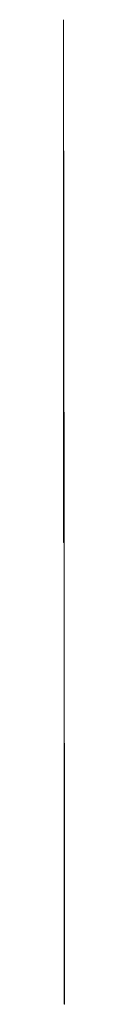
# Model space of a CAD drawing. Units: millimetres. Extents: x 0 to 2069, y 995 to 1695.
# Tile 1 of 2: x 0 to 0, y 1619 to 1695. Entities that reach past the tile are written whole.
import ezdxf

# ---------------------------------------------------------------- set-up
doc = ezdxf.new("R2010")
doc.units = ezdxf.units.MM
doc.layers.add('M-CONS', color=8, linetype='Continuous', lineweight=18)

msp = doc.modelspace()

# ---------------------------------------------------------------- linework, layer by layer
at = {"layer": 'M-CONS', "extrusion": (1, 0, 0)}
for p, q in [((-0.027, 1694.805, 555.349), (-0.027, 1694.805, 555.349)), ((-0.027, 1694.805, 555.349), (-0.027, 1654.805, 555.349)), ((0, 1654.805, 604.625), (-0.027, 1694.805, 555.349)), ((-0.027, 1654.805, 555.349), (0, 1654.805, 604.625))]:
    msp.add_line(p, q, dxfattribs=at)
at = {"layer": 'M-CONS'}
msp.add_polyline3d([(0, 1659.493, 547.71), (0, 1619.493, 547.71), (0.027, 1619.493, 596.986)], close=True, dxfattribs=at)

doc.saveas('drawing.dxf')
